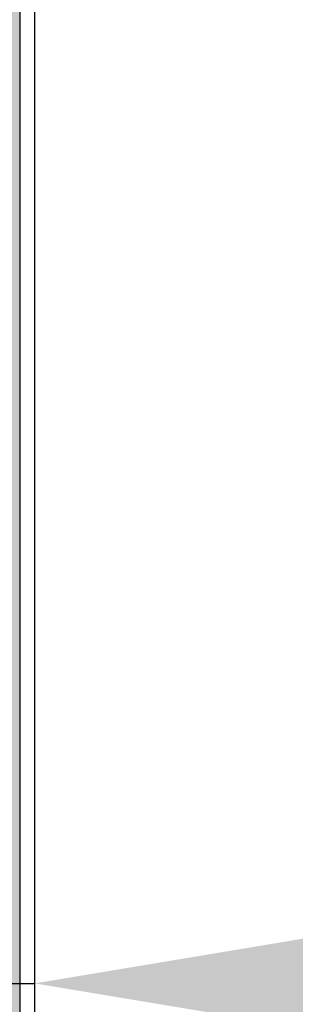
# Model space of a CAD drawing. Units: inches. Extents: x 2091 to 2899, y 967 to 2217.
# Tile 249 of 256: x 2212.144 to 2214.578, y 1139.939 to 1148.632. Entities that reach past the tile are written whole.
import ezdxf

# ---------------------------------------------------------------- set-up
doc = ezdxf.new("R2010")
doc.units = ezdxf.units.IN
doc.layers.add('A-ANNO-DIMS', color=2, linetype='Continuous', lineweight=18)
doc.layers.add('A-WALL-PATT', color=141, linetype='Continuous', lineweight=13, true_color=0xadddf7)
doc.styles.get("Standard").update_dxf_attribs({"font": 'arial.ttf'})
doc.dimstyles.new('ISO-25', dxfattribs={"dimtxt": 4, "dimasz": 4, "dimexe": 1.25, "dimexo": 0.625, "dimtad": 1, "dimdec": 0, "dimlunit": 3, "dimtxsty": 'Standard', "dimcen": 2.5, "dimadec": 0, "dimazin": 0, "dimtfac": 1, "dimtdec": 0, "dimtmove": 0, "dimatfit": 3, "dimfxl": 1, "dimarcsym": 0})

# ---------------------------------------------------------------- blocks, each defined once
blk = doc.blocks.new('*D37')
at = {"layer": 'A-ANNO-DIMS', "color": 0, "lineweight": -2, "transparency": 16777216}
for p, q in [((2203.1157, 1151.6221), (2203.1157, 1138.8736)), ((2212.2756, 1151.6221), (2212.2756, 1138.8736)), ((2199.1157, 1140.1236), (2195.1157, 1140.1236)), ((2203.1157, 1140.1236), (2212.2756, 1140.1236)), ((2216.2756, 1140.1236), (2245.9076, 1140.1236))]:
    blk.add_line(p, q, dxfattribs=at)
at = {"layer": 'A-ANNO-DIMS', "color": 0, "transparency": 16777216}
for points in [[(2199.1157, 1140.7902), (2199.1157, 1139.4569), (2203.1157, 1140.1236)], [(2216.2756, 1140.7902), (2216.2756, 1139.4569), (2212.2756, 1140.1236)]]:
    blk.add_solid(points, dxfattribs=at)
at = {"layer": 'Defpoints', "color": 0, "transparency": 16777216}
for p in [(2203.1157, 1152.2471), (2212.2756, 1152.2471), (2212.2756, 1140.1236)]:
    blk.add_point(p, dxfattribs=at)
at = {"layer": 'A-ANNO-DIMS', "color": 0, "transparency": 16777216, "insert": (2233.0916, 1142.7908), "char_height": 4, "attachment_point": 5}
blk.add_mtext('0\'-9" TYP.', dxfattribs=at)
blk = doc.blocks.new('*D71')
at = {"layer": 'A-ANNO-DIMS', "color": 0, "lineweight": -2, "transparency": 16777216}
for p, q in [((2212.1436, 1351.2941), (2212.1436, 969.4643)), ((2452.1436, 1351.2941), (2452.1436, 969.4643)), ((2216.1436, 970.7143), (2448.1436, 970.7143))]:
    blk.add_line(p, q, dxfattribs=at)
at = {"layer": 'A-ANNO-DIMS', "color": 0, "transparency": 16777216}
for points in [[(2216.1436, 971.381), (2216.1436, 970.0476), (2212.1436, 970.7143)], [(2448.1436, 971.381), (2448.1436, 970.0476), (2452.1436, 970.7143)]]:
    blk.add_solid(points, dxfattribs=at)
at = {"layer": 'Defpoints', "color": 0, "transparency": 16777216}
for p in [(2212.1436, 1351.9191), (2452.1436, 1351.9191), (2452.1436, 970.7143)]:
    blk.add_point(p, dxfattribs=at)
at = {"layer": 'A-ANNO-DIMS', "color": 0, "transparency": 16777216, "insert": (2332.1436, 973.3816), "char_height": 4, "attachment_point": 5}
blk.add_mtext('20\'-0"', dxfattribs=at)
blk = doc.blocks.new('*D75')
at = {"layer": 'A-ANNO-DIMS', "color": 0, "lineweight": -2, "transparency": 16777216}
for p, q in [((2212.1436, 1274.7941), (2212.1436, 969.4643)), ((2308.1436, 1274.7941), (2308.1436, 969.4643)), ((2216.1436, 970.7143), (2304.1436, 970.7143))]:
    blk.add_line(p, q, dxfattribs=at)
at = {"layer": 'A-ANNO-DIMS', "color": 0, "transparency": 16777216}
for points in [[(2216.1436, 971.381), (2216.1436, 970.0476), (2212.1436, 970.7143)], [(2304.1436, 971.381), (2304.1436, 970.0476), (2308.1436, 970.7143)]]:
    blk.add_solid(points, dxfattribs=at)
at = {"layer": 'Defpoints', "color": 0, "transparency": 16777216}
for p in [(2212.1436, 1275.4191), (2308.1436, 1275.4191), (2308.1436, 970.7143)]:
    blk.add_point(p, dxfattribs=at)
at = {"layer": 'A-ANNO-DIMS', "color": 0, "transparency": 16777216, "insert": (2260.1436, 973.3816), "char_height": 4, "attachment_point": 5}
blk.add_mtext('8\'-0"', dxfattribs=at)
blk = doc.blocks.new('*D91')
at = {"layer": 'A-ANNO-DIMS', "color": 0, "lineweight": -2, "transparency": 16777216}
for p, q in [((2211.6506, 1152.2471), (2098.3113, 1152.2471)), ((2099.5613, 1103.9191), (2099.5613, 1148.2471)), ((2211.5186, 1099.9191), (2098.3113, 1099.9191))]:
    blk.add_line(p, q, dxfattribs=at)
at = {"layer": 'A-ANNO-DIMS', "color": 0, "transparency": 16777216}
for points in [[(2098.8947, 1148.2471), (2100.228, 1148.2471), (2099.5613, 1152.2471)], [(2098.8947, 1103.9191), (2100.228, 1103.9191), (2099.5613, 1099.9191)]]:
    blk.add_solid(points, dxfattribs=at)
at = {"layer": 'Defpoints', "color": 0, "transparency": 16777216}
for p in [(2099.5613, 1152.2471), (2212.2756, 1152.2471), (2212.1436, 1099.9191)]:
    blk.add_point(p, dxfattribs=at)
at = {"layer": 'A-ANNO-DIMS', "color": 0, "transparency": 16777216, "insert": (2096.8681, 1126.0831), "char_height": 4, "attachment_point": 5, "rotation": 90}
blk.add_mtext('4\'-4 1/2"', dxfattribs=at)

msp = doc.modelspace()

# ---------------------------------------------------------------- hatches: boundary and pattern name
at = {"layer": 'A-WALL-PATT'}
h = msp.add_hatch(color=256, dxfattribs=at)
h.dxf.hatch_style = 1
h.paths.add_polyline_path([(2803.1436, 2050.9191), (2203.1436, 2050.9191), (2203.1436, 1090.9191), (2803.1436, 1090.9191)])
h.paths.add_polyline_path([(2635.7989, 1147.5405), (2674.5241, 1147.5405, 0.376086), (2678.5297, 1152.8802), (2678.5297, 1159.5565, 0.333335), (2674.5243, 1163.5618), (2674.5243, 1163.5619), (2674.5243, 1192.9344), (2635.806, 1192.9344), (2597.0876, 1192.9344), (2597.0876, 1163.5618, 0.333335), (2593.0823, 1159.5565), (2593.0823, 1152.8802, 0.376086), (2597.0879, 1147.5405)], flags=0)
h.paths.add_polyline_path([(2436.0104, 1278.2408, 0.000483), (2435.9526, 1278.215, -0.001328), (2435.9356, 1278.1117, -0.001711), (2436.1164, 1278.0408, 0.002185)], flags=0)
h.paths.add_polyline_path([(2794.1436, 1143.4191), (2794.1436, 1347.4191), (2543.3702, 1347.4191), (2543.3702, 1351.9191), (2794.1436, 1351.9191), (2794.1436, 1392.7136), (2793.9474, 1392.7136), (2793.9474, 1473.5369), (2794.1436, 1473.5369), (2794.1436, 1531.9191), (2650.1436, 1531.9191), (2650.1436, 1536.4191), (2794.1436, 1536.4191), (2794.1436, 1692.4191), (2609.3756, 1692.4191), (2609.3756, 1644.4191), (2604.8756, 1644.4191), (2604.8756, 1744.9191), (2609.3756, 1744.9191), (2609.3756, 1696.9191), (2794.1436, 1696.9191), (2794.1436, 1780.9191), (2609.6436, 1780.9191), (2493.8756, 1780.9191), (2493.8756, 1785.4191), (2609.6436, 1785.4191), (2794.1436, 1785.4191), (2794.1436, 1847.9388), (2793.9512, 1847.9388), (2793.9512, 1928.7622), (2794.1436, 1928.7622), (2794.1436, 1941.4191), (2614.1436, 1941.4191), (2614.1436, 1821.4191), (2609.6436, 1821.4191), (2609.6436, 1941.4191), (2392.1436, 1941.4191), (2392.1436, 1819.9191), (2387.6436, 1819.9191), (2387.6436, 1941.4191), (2212.1436, 1941.4191), (2212.1436, 1783.9191), (2392.1436, 1783.9191), (2392.1436, 1780.9191), (2212.1436, 1780.9191), (2212.1436, 1629.4191), (2387.6436, 1629.4191), (2387.6436, 1744.9191), (2392.1436, 1744.9191), (2392.1436, 1627.9191), (2317.1436, 1627.9191), (2317.1436, 1551.4191), (2317.1436, 1536.4191), (2459.3836, 1536.4191), (2459.3836, 1602.3965), (2463.8836, 1602.3965), (2463.8836, 1531.9191), (2456.6436, 1531.9191), (2456.6436, 1529.9191), (2452.1436, 1529.9191), (2452.1436, 1531.9191), (2312.6436, 1531.9191), (2312.6436, 1551.4191), (2306.1436, 1551.4191), (2306.1436, 1555.9191), (2308.1436, 1555.9191), (2308.1436, 1551.4191), (2312.6436, 1551.4191), (2312.6436, 1627.9191), (2212.1436, 1627.9191), (2212.1436, 1555.9191), (2270.1436, 1555.9191), (2270.1436, 1551.4191), (2212.1436, 1551.4191), (2212.1436, 1351.9191), (2272.1436, 1351.9191), (2272.1436, 1347.4191), (2212.1436, 1347.4191), (2212.1436, 1275.4191), (2308.1436, 1275.4191), (2308.1436, 1351.9191), (2452.1436, 1351.9191), (2452.1436, 1493.9191), (2456.6436, 1493.9191), (2456.6436, 1347.4191), (2312.6436, 1347.4191), (2312.6436, 1270.9191), (2212.1436, 1270.9191), (2212.1436, 1099.9191), (2281.2375, 1099.9191), (2282.871, 1110.9138), (2282.0083, 1116.9966), (2278.5577, 1121.4204), (2268.2056, 1128.0562), (2272.0876, 1128.0562), (2273.8129, 1131.927), (2279.4203, 1134.6919), (2285.0278, 1135.2449), (2287.6158, 1137.4568), (2288.0471, 1138.0098), (2289.3411, 1140.7747), (2291.0665, 1139.6687), (2292.3605, 1135.2449), (2295.3798, 1136.9038), (2296.2425, 1135.7979), (2297.1052, 1133.033), (2300.1246, 1138.0098), (2303.1439, 1138.0098), (2304.4379, 1135.7979), (2303.1439, 1133.586), (2306.5946, 1134.6919), (2307.8887, 1133.033), (2310.908, 1135.2449), (2313.9274, 1134.1389), (2315.6269, 1132.4271), (2308.32, 1117.5496), (2290.2038, 1109.8079), (2288.9098, 1103.1721), (2289.2723, 1099.9191), (2434.9182, 1099.9191), (2431.5932, 1124.7881), (2429.9302, 1169.5531), (2430.9272, 1240.5197), (2435.6589, 1238.1861), (2437.1352, 1196.5541), (2438.7982, 1143.9731), (2442.6782, 1111.9981), (2446.5582, 1099.9191), (2794.1436, 1099.9191), (2794.1436, 1138.9191), (2548.0324, 1138.9191), (2548.0324, 1143.4191), (2548.0324, 1148.8191), (2546.6685, 1148.0316), (2528.6857, 1179.1786, 0.256256), (2512.0324, 1148.8191), (2512.0324, 1143.4191), (2512.0324, 1138.9191), (2507.5324, 1138.9191), (2507.5324, 1143.4191), (2507.5324, 1148.8191, 0.256256), (2490.8792, 1179.1786), (2472.8964, 1148.0316), (2471.5324, 1148.8191), (2471.5324, 1143.4191), (2467.0324, 1143.4191), (2467.0324, 1269.9458, 0.039061), (2460.91, 1273.5801), (2467.0324, 1273.5801), (2467.0324, 1286.3254, 0.014511), (2465.2162, 1286.7619), (2467.0324, 1287.0526), (2467.0324, 1323.4191), (2471.5324, 1323.4191), (2471.5324, 1148.8191), (2489.5324, 1179.996), (2490.8964, 1179.2085), (2490.8792, 1179.1786, -0.256256), (2507.5324, 1148.8191), (2507.5324, 1143.4191), (2512.0324, 1143.4191), (2512.0324, 1148.8191, -0.256256), (2528.6857, 1179.1786), (2528.6685, 1179.2085), (2530.0324, 1179.996), (2548.0324, 1148.8191), (2548.0324, 1143.4191)], flags=16)
h.paths.add_polyline_path([(2607.7685, 1200.9451), (2607.7685, 1265.0306), (2597.0876, 1281.052), (2619.7846, 1281.052), (2627.7953, 1337.1269), (2635.7989, 1337.1269), (2643.8167, 1337.1269), (2651.8274, 1281.052), (2674.5243, 1281.052), (2663.8434, 1265.0306), (2663.8434, 1200.9451), (2635.806, 1200.9451)], flags=0)
edge = h.paths.add_edge_path(flags=0)
edge.add_ellipse((13303.8962, 1272.9987), major_axis=(-10595.313, 0), ratio=0.8423038701, start_angle=0.62823722, end_angle=0.6465541, ccw=False)
edge.add_ellipse((2711.7004, 1156.8527), major_axis=(2.2198, 0), ratio=0.842304, start_angle=111.53524, end_angle=180.62824, ccw=False)
edge.add_ellipse((13303.1563, 1272.9987), major_axis=(-10593.0263, 0), ratio=0.8423038695, start_angle=0.52827147, end_angle=0.6465541, ccw=False)
edge.add_line((2710.7646, 1175.3333), (2710.13, 1175.3333))
edge.add_ellipse((2710.13, 1176.5798), major_axis=(1.4798, 0), ratio=0.842304, start_angle=180, end_angle=270, ccw=False)
edge.add_line((2708.6501, 1176.5798), (2708.6501, 1200.7829))
edge.add_ellipse((2710.13, 1200.7829), major_axis=(1.4798, 0), ratio=0.842304, start_angle=90, end_angle=180, ccw=False)
edge.add_line((2710.13, 1202.0294), (2710.4651, 1202.0294))
edge.add_ellipse((13303.1563, 1272.9987), major_axis=(-10593.0263, 0), ratio=0.8423038695, start_angle=-0.09022909, end_angle=0.38386678, ccw=False)
edge.add_ellipse((2710.13, 1290.927), major_axis=(-1.4798, 0), ratio=0.842304, start_angle=0, end_angle=90, ccw=False)
edge.add_line((2708.6501, 1290.927), (2708.6501, 1315.1302))
edge.add_ellipse((2710.13, 1315.1302), major_axis=(-1.4798, 0), ratio=0.842304, start_angle=-90, end_angle=0, ccw=False)
edge.add_line((2710.13, 1316.3767), (2710.7063, 1316.3767))
edge.add_ellipse((3238.4017, 1296.2896), major_axis=(528.234, 0), ratio=0.84230387, start_angle=176.349572, end_angle=177.82005, ccw=False)
edge.add_ellipse((2775.063, 1071.4507), major_axis=(313.3078, 0), ratio=0.84230387, start_angle=102.125966, end_angle=103.780529, ccw=False)
edge.add_ellipse((2775.063, 1078.3057), major_axis=(-305.3029, 0), ratio=0.84230387, start_angle=-79.790461, end_angle=-77.555373, ccw=False)
edge.add_ellipse((2695.1418, 1541.9754), major_axis=(-250.9602, 0), ratio=0.84230387, start_angle=99.256566, end_angle=102.554933)
edge.add_line((2741.4103, 1334.2143), (2747.1325, 1337.3785))
edge.add_ellipse((2747.5386, 1336.8575), major_axis=(-0.7399, 0), ratio=0.842304, start_angle=270, end_angle=307.93313, ccw=False)
edge.add_ellipse((2747.5386, 1336.8575), major_axis=(-0.7399, 0), ratio=0.842304, start_angle=232.06687, end_angle=270, ccw=False)
edge.add_line((2747.9447, 1337.3785), (2753.6669, 1334.2143))
edge.add_ellipse((2799.9355, 1541.9754), major_axis=(250.9602, 0), ratio=0.84230387, start_angle=257.445067, end_angle=260.743434)
edge.add_ellipse((2720.0142, 1078.3057), major_axis=(305.3029, 0), ratio=0.84230387, start_angle=77.555373, end_angle=79.790461, ccw=False)
edge.add_ellipse((2720.0142, 1071.4507), major_axis=(-313.3078, 0), ratio=0.84230387, start_angle=256.219471, end_angle=257.874034, ccw=False)
edge.add_ellipse((2256.6755, 1296.2896), major_axis=(-528.234, 0), ratio=0.84230387, start_angle=182.17995, end_angle=183.650428, ccw=False)
edge.add_line((2784.3709, 1316.3767), (2784.9472, 1316.3767))
edge.add_ellipse((2784.9472, 1315.1302), major_axis=(1.4798, 0), ratio=0.842304, start_angle=0, end_angle=90, ccw=False)
edge.add_line((2786.4271, 1315.1302), (2786.4271, 1290.927))
edge.add_ellipse((2784.9472, 1290.927), major_axis=(1.4798, 0), ratio=0.842304, start_angle=270, end_angle=360, ccw=False)
edge.add_ellipse((-7808.0791, 1272.9987), major_axis=(10593.0263, 0), ratio=0.8423038695, start_angle=-0.38386678, end_angle=0.09022909, ccw=False)
edge.add_line((2784.6122, 1202.0294), (2784.9472, 1202.0294))
edge.add_ellipse((2784.9472, 1200.7829), major_axis=(1.4798, 0), ratio=0.842304, start_angle=0, end_angle=90, ccw=False)
edge.add_line((2786.4271, 1200.7829), (2786.4271, 1176.5798))
edge.add_ellipse((2784.9472, 1176.5798), major_axis=(-1.4798, 0), ratio=0.842304, start_angle=90, end_angle=180, ccw=False)
edge.add_line((2784.9472, 1175.3333), (2784.3126, 1175.3333))
edge.add_ellipse((-7808.0791, 1272.9987), major_axis=(10593.0263, 0), ratio=0.8423038695, start_angle=-0.6186432, end_angle=-0.52827147, ccw=False)
edge.add_ellipse((2783.3768, 1156.8527), major_axis=(-2.2198, 0), ratio=0.842304, start_angle=179.37176, end_angle=248.46476, ccw=False)
edge.add_ellipse((-7808.819, 1272.9987), major_axis=(-10595.313, 0), ratio=0.8423038658, start_angle=179.35344592, end_angle=179.3717628, ccw=False)
edge.add_ellipse((2780.2973, 1153.5008), major_axis=(-5.2464, 0), ratio=0.842304, start_angle=90, end_angle=179.35345, ccw=False)
edge.add_line((2780.2973, 1149.0817), (2714.7799, 1149.0817))
edge.add_ellipse((2714.7799, 1153.5008), major_axis=(5.2464, 0), ratio=0.842304, start_angle=180.64655, end_angle=270, ccw=False)
edge = h.paths.add_edge_path(flags=0)
edge.add_line((2718.1874, 1151.0078), (2718.1874, 1170.4724))
edge.add_ellipse((2721.1471, 1170.4724), major_axis=(-2.9597, 0), ratio=0.842304, start_angle=-90, end_angle=0, ccw=False)
edge.add_line((2721.1471, 1172.9653), (2773.9302, 1172.9653))
edge.add_ellipse((2773.9302, 1170.4724), major_axis=(-2.9597, 0), ratio=0.842304, start_angle=180, end_angle=270, ccw=False)
edge.add_line((2776.8899, 1170.4724), (2776.8899, 1151.0078))
edge.add_line((2776.8899, 1151.0078), (2718.1874, 1151.0078))
edge = h.paths.add_edge_path(flags=0)
edge.add_line((2718.1874, 1180.2342), (2718.1874, 1199.0578))
edge.add_ellipse((2747.5386, 1320.3986), major_axis=(147.0179, 0), ratio=0.84230387, start_angle=256.401865, end_angle=283.598135)
edge.add_line((2776.8899, 1199.0578), (2776.8899, 1180.2342))
edge.add_ellipse((2747.5386, 1301.575), major_axis=(147.0179, 0), ratio=0.84230387, start_angle=256.401865, end_angle=283.598135, ccw=False)
edge = h.paths.add_edge_path(flags=0)
edge.add_ellipse((13303.1563, 1272.9987), major_axis=(-10591.5465, 0), ratio=0.8423038696, start_angle=0.05559431, end_angle=0.37776419, ccw=False)
edge.add_line((2711.6169, 1262.7217), (2715.6674, 1249.4954))
edge.add_ellipse((6413.892, 1241.6919), major_axis=(-3698.2362, 0), ratio=0.84230387, start_angle=-0.1208974, end_angle=0.3640763)
edge.add_line((2715.761, 1218.1925), (2711.9343, 1203.1674))
edge = h.paths.add_edge_path(flags=0)
edge.add_line((2718.1874, 1251.0746), (2716.0025, 1267.4504))
edge.add_ellipse((2742.1512, 1202.1895), major_axis=(81.7726, 0), ratio=0.8423039, start_angle=94.277421, end_angle=111.834954, ccw=False)
edge.add_line((2737.0097, 1270.9306), (2758.0675, 1270.9306))
edge.add_ellipse((2752.9261, 1202.1895), major_axis=(81.7726, 0), ratio=0.8423039, start_angle=68.165046, end_angle=85.722579, ccw=False)
edge.add_line((2779.0747, 1267.4504), (2776.8899, 1251.0746))
edge.add_ellipse((2750.3381, 1187.8854), major_axis=(79.5797, 0), ratio=0.8423039, start_angle=67.208085, end_angle=85.12993)
edge.add_line((2756.0347, 1254.7437), (2739.0426, 1254.7437))
edge.add_ellipse((2744.7392, 1187.8854), major_axis=(79.5797, 0), ratio=0.8423039, start_angle=94.87007, end_angle=112.791915)
edge = h.paths.add_edge_path(flags=0)
edge.add_line((2783.1429, 1203.1674), (2779.3162, 1218.1925))
edge.add_ellipse((-918.8147, 1241.6919), major_axis=(3698.2362, 0), ratio=0.84230387, start_angle=-0.3640763, end_angle=0.1208974)
edge.add_line((2779.4098, 1249.4954), (2783.4604, 1262.7217))
edge.add_ellipse((-7808.0791, 1272.9987), major_axis=(-10591.5465, 0), ratio=0.8423038695, start_angle=179.62223581, end_angle=179.94440569, ccw=False)
edge = h.paths.add_edge_path(flags=0)
edge.add_ellipse((2734.2009, 1286.6904), major_axis=(-0.3566, 6.3401), ratio=0.603834, start_angle=89.00201, end_angle=253.65741, ccw=False)
edge.add_line((2730.369, 1286.5418), (2730.369, 1301.352))
edge.add_line((2730.369, 1301.352), (2735.9133, 1305.2148))
edge.add_ellipse((2736.3849, 1304.7346), major_axis=(0.7399, 0), ratio=0.842304, start_angle=90, end_angle=134.48021, ccw=False)
edge.add_line((2736.3849, 1305.3578), (2738.0328, 1305.3578))
edge.add_line((2738.0328, 1305.3578), (2738.0328, 1307.7079))
edge.add_ellipse((2794.2016, 1307.7079), major_axis=(56.1689, 0), ratio=0.8423039, start_angle=150.56143, end_angle=180, ccw=False)
edge.add_ellipse((2700.8756, 1307.7079), major_axis=(-56.1689, 0), ratio=0.8423039, start_angle=180, end_angle=209.43857, ccw=False)
edge.add_line((2757.0444, 1307.7079), (2757.0444, 1305.3578))
edge.add_line((2757.0444, 1305.3578), (2758.6923, 1305.3578))
edge.add_ellipse((2758.6923, 1304.7346), major_axis=(-0.7399, 0), ratio=0.842304, start_angle=225.51979, end_angle=270, ccw=False)
edge.add_line((2759.1639, 1305.2148), (2764.7082, 1301.352))
edge.add_line((2764.7082, 1301.352), (2764.7082, 1286.5418))
edge.add_ellipse((2760.8763, 1286.6904), major_axis=(0.3566, 6.3401), ratio=0.603834, start_angle=106.34259, end_angle=270.99799, ccw=False)
edge.add_line((2757.0444, 1285.7971), (2757.0444, 1307.7079))
edge.add_ellipse((2700.8756, 1307.7079), major_axis=(-56.1689, 0), ratio=0.8423039, start_angle=180, end_angle=209.43857)
edge.add_ellipse((2794.2016, 1307.7079), major_axis=(56.1689, 0), ratio=0.8423039, start_angle=150.56143, end_angle=180)
edge.add_line((2738.0328, 1307.7079), (2738.0328, 1285.7971))
h.paths.add_polyline_path([(2417.8123, 1104.4497), (2413.4923, 1102.5297), (2410.6123, 1103.9697), (2409.1723, 1106.3697), (2407.2523, 1107.3297), (2406.2923, 1109.7297), (2405.3323, 1114.0497), (2405.3323, 1117.8897), (2406.2923, 1120.1297), (2407.2523, 1119.8097), (2408.8483, 1118.3277), (2410.1739, 1119.4242), (2410.2113, 1120.4057), (2411.0407, 1121.4191), (2410.6993, 1119.8587), (2410.1739, 1119.4242), (2410.0885, 1117.1761), (2411.1328, 1116.2063), (2413.9723, 1119.3297), (2416.8523, 1120.7697), (2416.8697, 1120.7988), (2417.0351, 1119.4051), (2417.8962, 1118.1434), (2418.2923, 1118.3697), (2419.5444, 1120.0393), (2419.3609, 1118.3875), (2419.0321, 1119.3562), (2418.3989, 1118.5119), (2419.2523, 1114.5297), (2418.7941, 1107.1988)], flags=0)
h.paths.add_polyline_path([(2508.8702, 1347.4191), (2508.3702, 1347.4191), (2508.3702, 1351.9191), (2508.8702, 1351.9191)], flags=0)
h.paths.add_polyline_path([(2473.3702, 1347.4191), (2472.3702, 1347.4191), (2467.8702, 1347.4191), (2467.8702, 1455.4191), (2472.3702, 1455.4191), (2472.3702, 1352.4191), (2473.3702, 1352.4191)], flags=0)
h.paths.add_polyline_path([(2352.1062, 1217.4462), (2349.2262, 1218.8862), (2347.7862, 1221.2862), (2345.8662, 1222.2462), (2344.9062, 1224.6462), (2343.9462, 1228.9662), (2343.9462, 1232.8062), (2344.9062, 1235.0462), (2345.8662, 1234.7262), (2347.4623, 1233.2442), (2348.7879, 1234.3407), (2348.8252, 1235.3222), (2349.6547, 1236.3355), (2349.3132, 1234.7752), (2348.7879, 1234.3407), (2348.7024, 1232.0926), (2349.7468, 1231.1228), (2352.5862, 1234.2462), (2355.4662, 1235.6862), (2355.4837, 1235.7153), (2355.649, 1234.3216), (2356.5102, 1233.0599), (2356.9062, 1233.2862), (2358.1584, 1234.9558), (2357.9749, 1233.304), (2357.6461, 1234.2726), (2357.0129, 1233.4284), (2357.8662, 1229.4462), (2357.4081, 1222.1153), (2356.4262, 1219.3662)], flags=0)
h.paths.add_polyline_path([(2348.2968, 1112.2244), (2347.0138, 1112.3104), (2345.5298, 1114.1274), (2345.7318, 1115.8584), (2346.8118, 1116.9824), (2346.8118, 1114.6464), (2345.8668, 1114.2144), (2346.8798, 1114.3004)], flags=0)
h.paths.add_polyline_path([(2347.0138, 1110.9264), (2346.2718, 1110.4934), (2346.6098, 1111.1864)], flags=0)
h.paths.add_polyline_path([(2345.8668, 1118.1944), (2345.5298, 1117.3294), (2343.7078, 1118.0214), (2344.3828, 1118.6264)], flags=0)
h.paths.add_polyline_path([(2346.6768, 1109.2824), (2346.0698, 1108.0714), (2345.8668, 1110.0614)], flags=0)
h.paths.add_polyline_path([(2345.0568, 1119.7514), (2343.6398, 1119.7514), (2343.9778, 1121.1354)], flags=0)
h.paths.add_polyline_path([(2345.2598, 1116.5504), (2345.1248, 1115.8584), (2344.9218, 1115.6854), (2344.7198, 1116.3774)], flags=0)
h.paths.add_polyline_path([(2345.6648, 1112.3104), (2345.4618, 1111.5324), (2344.0448, 1111.9644), (2344.6518, 1112.5704)], flags=0)
h.paths.add_polyline_path([(2345.1918, 1113.3494), (2344.4498, 1113.8684), (2344.7198, 1114.3874)], flags=0)
h.paths.add_polyline_path([(2344.6518, 1116.8094), (2344.1798, 1115.6854), (2344.6518, 1115.3394), (2343.9098, 1114.9064), (2343.0328, 1115.9444), (2343.6398, 1116.4634)], flags=0)
h.paths.add_polyline_path([(2345.8668, 1106.6864), (2344.9898, 1105.5624), (2344.5168, 1106.6004)], flags=0)
h.paths.add_polyline_path([(2344.8548, 1110.0614), (2344.5168, 1109.2824), (2344.1128, 1109.7154)], flags=0)
h.paths.add_polyline_path([(2344.0448, 1113.5224), (2343.4378, 1113.0894), (2342.7628, 1113.9544)], flags=0)
h.paths.add_polyline_path([(2344.3148, 1111.0124), (2342.9648, 1110.3204), (2342.9648, 1111.0994)], flags=0)
h.paths.add_polyline_path([(2345.1248, 1104.6974), (2344.5848, 1103.7454), (2344.4498, 1104.2644)], flags=0)
h.paths.add_polyline_path([(2342.8298, 1121.2224), (2341.7498, 1120.5304), (2340.5358, 1121.0494), (2340.1308, 1121.8284), (2340.6708, 1122.9524), (2341.1428, 1121.8284), (2341.6148, 1122.0014)], flags=0)
h.paths.add_polyline_path([(2342.9648, 1119.7514), (2343.0328, 1118.4534), (2342.0878, 1118.0214), (2342.0198, 1119.4914)], flags=0)
h.paths.add_polyline_path([(2342.6948, 1116.8964), (2341.9528, 1116.6364), (2342.0198, 1117.3294)], flags=0)
h.paths.add_polyline_path([(2343.0328, 1112.2244), (2342.0198, 1111.7914), (2341.5478, 1112.2244), (2342.3578, 1113.3494)], flags=0)
h.paths.add_polyline_path([(2343.7748, 1104.4374), (2342.6278, 1102.8804), (2342.6948, 1104.6104), (2343.4378, 1105.1294)], flags=0)
h.paths.add_polyline_path([(2342.0198, 1115.0794), (2340.8058, 1115.5124), (2340.9408, 1116.3774)], flags=0)
h.paths.add_polyline_path([(2341.4808, 1120.0974), (2341.4808, 1119.4054), (2341.0758, 1119.5784), (2341.1428, 1120.0974)], flags=0)
h.paths.add_polyline_path([(2341.8178, 1114.4734), (2340.9408, 1113.0894), (2340.8058, 1114.5604)], flags=0)
h.paths.add_polyline_path([(2341.1428, 1118.5404), (2340.9408, 1116.9824), (2339.0508, 1117.6754), (2339.0508, 1118.6264)], flags=0)
h.paths.add_polyline_path([(2342.6948, 1101.6684), (2341.9528, 1101.8414), (2342.5598, 1102.3614)], flags=0)
h.paths.add_polyline_path([(2340.3328, 1119.6654), (2338.4438, 1119.5784), (2337.9038, 1120.3574), (2339.6578, 1120.6164)], flags=0)
h.paths.add_polyline_path([(2340.3328, 1115.3394), (2340.0628, 1113.6954), (2339.3878, 1115.3394)], flags=0)
h.paths.add_polyline_path([(2341.8178, 1103.8314), (2341.5478, 1102.8804), (2341.1428, 1103.6584)], flags=0)
h.paths.add_polyline_path([(2339.0508, 1122.8664), (2337.2958, 1121.8284), (2337.0938, 1123.1254), (2337.7688, 1123.8184)], flags=0)
h.paths.add_polyline_path([(2339.1178, 1121.7414), (2338.8478, 1121.2224), (2338.1738, 1121.0494), (2338.3758, 1121.5684)], flags=0)
h.paths.add_polyline_path([(2339.1858, 1119.3194), (2338.6458, 1118.7134), (2338.2408, 1118.1074), (2338.2408, 1118.8864)], flags=0)
h.paths.add_polyline_path([(2341.1428, 1101.9284), (2340.6028, 1101.2364), (2340.0628, 1101.8414), (2340.6028, 1102.3614)], flags=0)
h.paths.add_polyline_path([(2337.6338, 1117.7614), (2336.6208, 1118.2804), (2337.2958, 1118.9724)], flags=0)
h.paths.add_polyline_path([(2336.8238, 1119.5784), (2334.7988, 1118.9724), (2335.2038, 1120.3574), (2336.5538, 1120.8764)], flags=0)
h.paths.add_polyline_path([(2339.1178, 1100.4574), (2337.3638, 1100.5434), (2336.7558, 1101.2364)], flags=0)
h.paths.add_polyline_path([(2336.3508, 1122.4334), (2336.0138, 1121.9144), (2334.9338, 1122.4334), (2334.5288, 1123.4714), (2335.7438, 1122.7794)], flags=0)
h.paths.add_polyline_path([(2334.7318, 1120.8764), (2334.2588, 1120.3574), (2334.0568, 1120.7894), (2334.5968, 1121.3084)], flags=0)
h.paths.add_polyline_path([(2334.4618, 1122.1744), (2332.5718, 1121.3084), (2331.3568, 1122.1744), (2332.0998, 1122.8664)], flags=0)
h.paths.add_polyline_path([(2334.2588, 1118.5404), (2333.3818, 1118.4534), (2333.6518, 1119.3194)], flags=0)
h.paths.add_polyline_path([(2335.5418, 1102.2744), (2334.1918, 1102.6204), (2335.2718, 1103.3124)], flags=0)
h.paths.add_polyline_path([(2332.7068, 1119.6654), (2331.6948, 1120.4434), (2332.5048, 1120.7894)], flags=0)
h.paths.add_polyline_path([(2334.7318, 1101.1494), (2333.5168, 1101.5824), (2333.9888, 1101.7554)], flags=0)
h.paths.add_polyline_path([(2332.6398, 1116.6364), (2331.0868, 1116.2904), (2331.9648, 1118.1944)], flags=0)
h.paths.add_polyline_path([(2330.7498, 1121.5684), (2330.2768, 1120.2704), (2328.5228, 1119.3194), (2328.9948, 1121.0494)], flags=0)
h.paths.add_polyline_path([(2330.7498, 1118.6264), (2330.0078, 1117.5024), (2329.8728, 1118.0214)], flags=0)
h.paths.add_polyline_path([(2332.0998, 1102.3614), (2330.5468, 1102.0144), (2331.6948, 1102.9664)], flags=0)
h.paths.add_polyline_path([(2329.5348, 1113.6084), (2329.0628, 1112.3104), (2328.5898, 1113.3494)], flags=0)
h.paths.add_polyline_path([(2328.3878, 1117.8484), (2327.5098, 1116.5504), (2327.1728, 1117.7614)], flags=0)
h.paths.add_polyline_path([(2329.7378, 1106.5134), (2329.5348, 1105.3024), (2328.2528, 1106.0814)], flags=0)
h.paths.add_polyline_path([(2328.6578, 1114.3874), (2328.0498, 1114.1274), (2328.3198, 1114.9064)], flags=0)
h.paths.add_polyline_path([(2328.3198, 1112.2244), (2327.1058, 1112.1374), (2326.7008, 1112.6564)], flags=0)
h.paths.add_polyline_path([(2326.9028, 1115.2524), (2326.7008, 1114.1274), (2325.2158, 1113.6084), (2326.0928, 1115.3394)], flags=0)
h.paths.add_polyline_path([(2326.6328, 1108.3304), (2326.0928, 1107.3794), (2325.8908, 1108.5034), (2326.4978, 1109.1094)], flags=0)
h.paths.add_polyline_path([(2615.1436, 1531.9191), (2609.6436, 1531.9191), (2609.6436, 1620.4191), (2614.1436, 1620.4191), (2614.1436, 1536.4191), (2615.1436, 1536.4191)], flags=0)
h.paths.add_polyline_path([(2545.1436, 1563.4191), (2464.1436, 1563.4191), (2464.1436, 1632.4191), (2509.1436, 1632.4191), (2509.1436, 1627.9191), (2509.1436, 1603.9191), (2468.6436, 1603.9191), (2468.6436, 1567.9191), (2540.6436, 1567.9191), (2540.6436, 1591.9191), (2545.1436, 1591.9191)], flags=0)
h.paths.add_polyline_path([(2388.969, 1549.9857), (2357.4342, 1549.9857), (2357.4342, 1623.3608), (2399.3628, 1623.3608), (2435.6895, 1623.3608), (2435.5925, 1602.5593), (2435.5925, 1602.3965), (2388.969, 1602.3965)], flags=0)
h.paths.add_polyline_path([(2388.8806, 1555.8092), (2374.9044, 1555.8092), (2374.9044, 1600.5716), (2374.9044, 1615.4576), (2406.3509, 1615.4576), (2406.3509, 1618.9394), (2412.1743, 1615.4576), (2406.3509, 1611.9759), (2406.3509, 1615.4576), (2388.8806, 1615.4576)], flags=0)
h.paths.add_polyline_path([(2568.8756, 1644.4191), (2453.3756, 1644.4191), (2453.3756, 1785.4191), (2457.8756, 1785.4191), (2457.8756, 1648.9191), (2568.8756, 1648.9191)], flags=0)
h.paths.add_polyline_path([(2212.1436, 1945.9191), (2212.1436, 2041.9191), (2794.1436, 2041.9191), (2794.1436, 1945.9191)], flags=16)
h.paths.add_polyline_path([(2271.0827, 1964.3172), (2776.853, 1964.3172), (2776.853, 2037.1696), (2271.0827, 2037.1696)], flags=8)
h.paths.add_polyline_path([(2380.6493, 1536.8241), (2461.0408, 1536.8241), (2461.0408, 1554.6526), (2380.6493, 1554.6526)], flags=8)
h.paths.add_polyline_path([(2240.7557, 1609.7255), (2309.1858, 1609.7255), (2309.1858, 1617.6982), (2240.7557, 1617.6982)], flags=8)
h.paths.add_polyline_path([(2212.6773, 1313.5041), (2282.5915, 1313.5041), (2282.5915, 1322.7452), (2212.6773, 1322.7452)], flags=8)
h.paths.add_polyline_path([(2457.112, 1114.7786), (2558.4816, 1114.7786), (2558.4816, 1142.2197), (2457.112, 1142.2197)], flags=8)
h.paths.add_polyline_path([(2473.4423, 1273.0101), (2604.6412, 1273.0101), (2604.6412, 1318.3469), (2473.4423, 1318.3469)], flags=8)
h.paths.add_polyline_path([(2638.8763, 1626.9774), (2684.2504, 1627.9767), (2684.0385, 1637.5975), (2638.6644, 1636.5982)], flags=8)
h.paths.add_polyline_path([(2537.5906, 1453.7934), (2628.3895, 1453.7934), (2628.3895, 1475.3448), (2537.5906, 1475.3448)], flags=8)
h.paths.add_polyline_path([(2504.1376, 1714.6324), (2554.6472, 1714.6324), (2554.6472, 1730.2377), (2504.1376, 1730.2377)], flags=8)
h.paths.add_polyline_path([(2487.5012, 1575.6519), (2535.0971, 1575.6519), (2535.0971, 1598.3776), (2487.5012, 1598.3776)], flags=8)
h.paths.add_polyline_path([(2709.0994, 1735.7103), (2740.0166, 1735.7103), (2740.0166, 1749.9376), (2709.0994, 1749.9376)], flags=8)
h.paths.add_polyline_path([(2442.4384, 1792.1717), (2564.7288, 1792.1717), (2564.7288, 1842.0002), (2442.4384, 1842.0002)], flags=8)
h.paths.add_polyline_path([(2655.8158, 1809.6441), (2789.5201, 1806.6938), (2790.085, 1832.2916), (2656.3806, 1835.2419)], flags=8)
h.paths.add_polyline_path([(2234.8427, 1797.7201), (2368.5929, 1794.7689), (2369.1607, 1820.5041), (2235.4106, 1823.4554)], flags=8)
h.paths.add_polyline_path([(2245.1385, 1644.0063), (2398.4277, 1640.6239), (2398.9948, 1666.3248), (2245.7056, 1669.7073)], flags=8)
h.paths.add_polyline_path([(2306.1428, 1431.1685), (2413.7683, 1428.7937), (2414.3331, 1454.3915), (2306.7077, 1456.7664)], flags=8)
h.paths.add_polyline_path([(2306.8346, 1458.2331), (2393.3805, 1456.3234), (2393.9328, 1481.3544), (2307.3869, 1483.2641)], flags=8)

# ---------------------------------------------------------------- dimensions: what is measured, and where the dimension line sits
at = {"layer": 'A-ANNO-DIMS'}
for base, p1, p2, picture, middle in [((2452.1436, 970.7143), (2212.1436, 1351.9191), (2452.1436, 1351.9191), '*D71', (2332.1436, 973.3816)), ((2308.1436, 970.7143), (2212.1436, 1275.4191), (2308.1436, 1275.4191), '*D75', (2260.1436, 973.3816))]:
    dim = msp.add_linear_dim(base=base, p1=p1, p2=p2, dimstyle='ISO-25', override={"dimdec": 1, "dimlfac": 1, "dimrnd": 0, "dimzin": 1, "dimdsep": 46, "dimlunit": 4, "dimfrac": 2}, dxfattribs=at)
    dim.commit()
    dim.dimension.update_dxf_attribs({"geometry": picture, "text_midpoint": middle})
dim = msp.add_linear_dim(base=(2099.5613, 1152.2471), p1=(2212.1436, 1099.9191), p2=(2212.2756, 1152.2471), angle=90, dimstyle='ISO-25', override={"dimdec": 1, "dimlfac": 1, "dimrnd": 0, "dimzin": 1, "dimdsep": 46, "dimlunit": 4, "dimfrac": 2}, dxfattribs=at)
dim.commit()
dim.dimension.update_dxf_attribs({"geometry": '*D91', "text_midpoint": (2096.8681, 1126.0831)})
dim = msp.add_linear_dim(base=(2212.2756, 1140.1236), p1=(2203.1157, 1152.2471), p2=(2212.2756, 1152.2471), text='<> TYP.', dimstyle='ISO-25', override={"dimdec": 1, "dimlfac": 1, "dimrnd": 0, "dimzin": 1, "dimdsep": 46, "dimlunit": 4, "dimfrac": 2}, dxfattribs=at)
dim.commit()
dim.dimension.update_dxf_attribs({"geometry": '*D37', "text_midpoint": (2233.0916, 1142.7908)})

doc.saveas('drawing.dxf')
